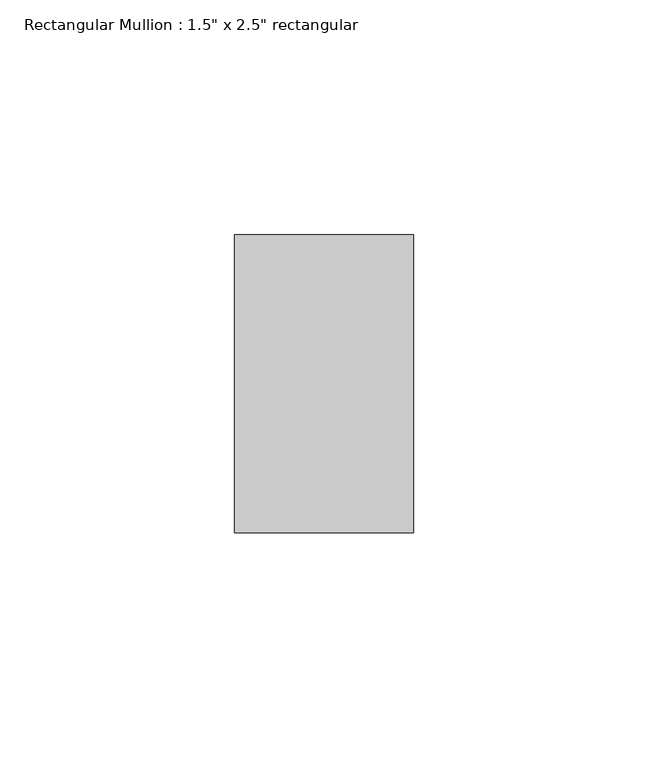
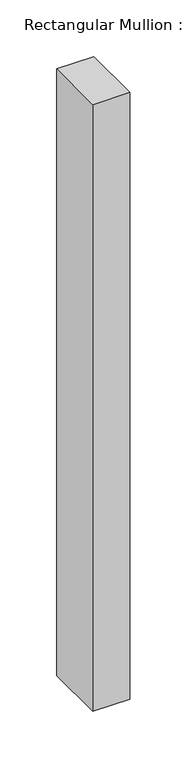
"""IFC4 building model written with IfcOpenShell, lengths in millimetres: member geometry."""

from ifc_helpers import new_model, si_unit, frame, origin, place, context, project, spatial, polyline, outline, extrude, source, transform, mapped, element, save


def member_92f0adee(model_context):
    return source(origin(), model_context, "Body", "SweptSolid", [
        extrude(outline(polyline([(0.0, 31.75), (0.0, -31.75), (-38.1, -31.75), (-38.1, 31.75), (0.0, 31.75)])), frame((0.0, 0.0, -654.05), z_axis=(0.0, 0.0, 1.0), x_axis=(1.0, 0.0, 0.0)), (0.0, 0.0, 1.0), 654.05),
    ])


if __name__ == "__main__":
    model = new_model("IFC4")
    model_context = context("Model", 3, world=origin())
    ifc_project = project(units=[si_unit("LENGTHUNIT", "METRE", prefix="MILLI")], contexts=[model_context])
    site = spatial("IfcSite", under=ifc_project)
    building = spatial("IfcBuilding", under=site)
    placement = place(None, origin())
    member_shape = member_92f0adee(model_context)
    element("IfcMember", 1, ObjectType="Rectangular Mullion : 1.5\" x 2.5\" rectangular", at=placement, inside=building, context=model_context, shape_type="MappedRepresentation", body=[
        mapped(member_shape, transform((0.0, 0.0, 0.0), x_axis=(1.0, 0.0, 0.0), y_axis=(0.0, 1.0, 0.0), z_axis=(0.0, 0.0, 1.0))),
    ])
    save(model, "model.ifc")

# Revit data of these elements
# Type "Rectangular Mullion : 1.5\" x 2.5\" rectangular"
#   built-in parameter 1007304 = 0.208333 (stored number, unit not read)
#   built-in parameter 1007301 = 0.0625 (stored number, unit not read)
#   built-in parameter 1007300 = 0.0625 (stored number, unit not read)
# Element 1 (IfcMember, "Rectangular Mullion : 1.5\" x 2.5\" rectangular")
#   Materials on its faces: "Leather - Black"
# Materials
#   "Leather - Black": class "Generic", colour RGB 40 40 40, transparency 0, Cost = 0
